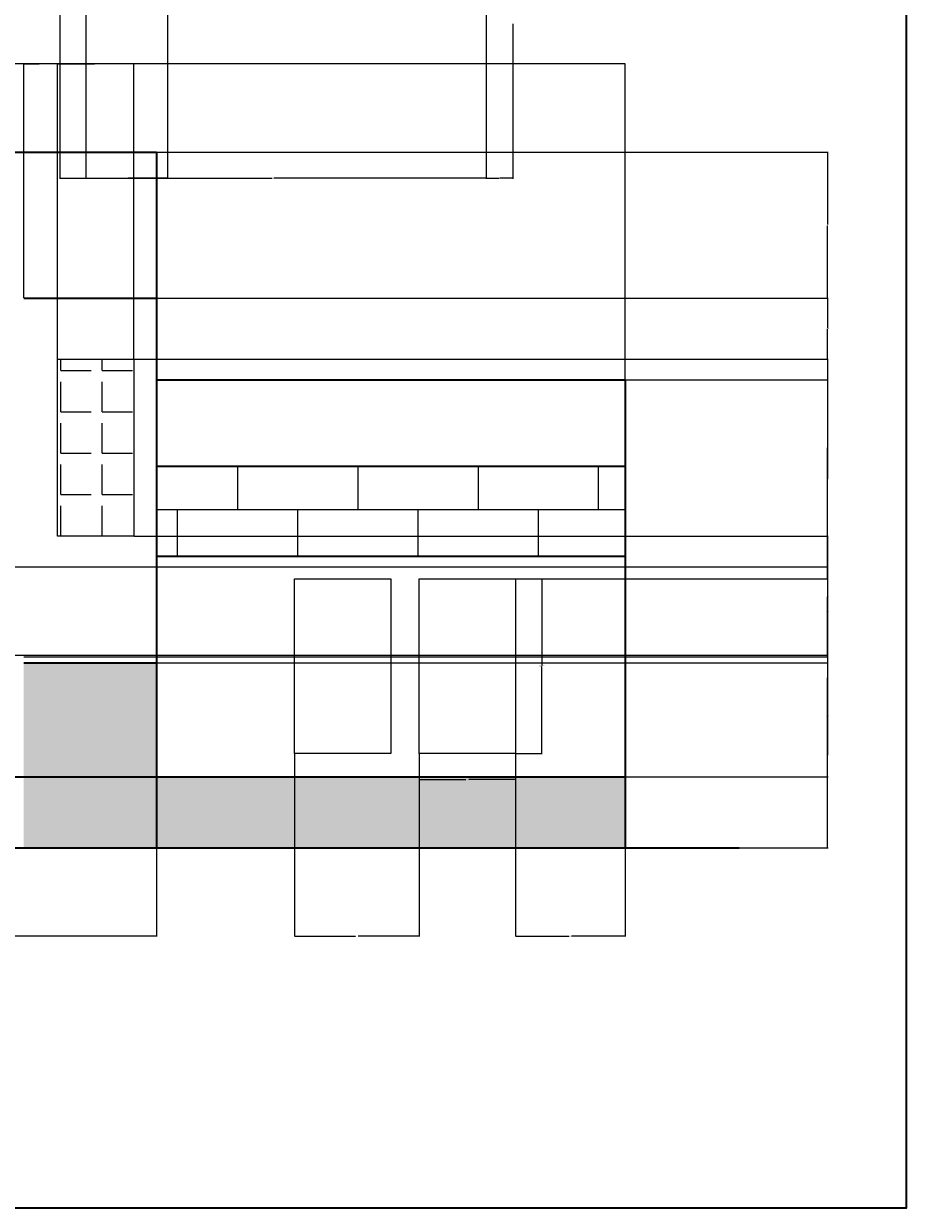
# Model space of a CAD drawing. Units: feet. Extents: x 3406 to 4127, y 2162 to 3204.
# Tile 2 of 3: x 3829 to 4127, y 2162 to 2562. Entities that reach past the tile are written whole.
import ezdxf

# ---------------------------------------------------------------- set-up
doc = ezdxf.new("R2010")
doc.units = ezdxf.units.FT
for name, color, linetype, lineweight in [('A-ANNO-DIMS', 2, 'Continuous', 18), ('A-ANNO-TTLB', 7, 'Continuous', 35), ('A-ELEV', 7, 'Continuous', 35), ('A-ELEV-GRND', 7, 'Continuous', 35), ('A-ELEV-PATT', 8, 'Continuous', 13), ('A-GLAZ', 4, 'Continuous', 25), ('A-GLAZ-PATT', 9, 'Continuous', 13)]:
    doc.layers.add(name, color=color, linetype=linetype, lineweight=lineweight)
doc.styles.get("Standard").update_dxf_attribs({"font": 'arial.ttf'})
doc.dimstyles.get("Standard").update_dxf_attribs({"dimtxt": 0.18, "dimasz": 0.18, "dimexe": 0.18, "dimexo": 0.0625, "dimgap": 0.09, "dimtad": 0, "dimtih": 1, "dimtoh": 1, "dimdec": 4, "dimzin": 0, "dimdsep": 46, "dimtxsty": 'Standard', "dimcen": 0.09, "dimadec": 0, "dimazin": 0, "dimtfac": 1, "dimtdec": 4, "dimtofl": 0, "dimtmove": 0, "dimatfit": 3, "dimfxl": 1, "dimtolj": 1, "dimtzin": 0, "dimarcsym": 0})

# ---------------------------------------------------------------- blocks, each defined once
blk = doc.blocks.new('WIN-ELEV-SINGLE')
blk.add_lwpolyline([(0, 59.01), (32.53, 59.01), (32.53, 0), (0, 0)], close=True)
blk = doc.blocks.new('*D2')
at = {"layer": 'A-ANNO-DIMS', "color": 0, "lineweight": -2, "transparency": 16777216}
for p, q in [((3995.35, 2374.42), (4004.32, 2374.42)), ((4004.14, 2374.24), (4004.14, 2345.1)), ((4004.14, 2315.6), (4004.14, 2344.74)), ((3995.35, 2315.42), (4004.32, 2315.42))]:
    blk.add_line(p, q, dxfattribs=at)
at = {"layer": 'A-ANNO-DIMS', "color": 0, "transparency": 16777216}
for points in [[(4004.11, 2374.24), (4004.17, 2374.24), (4004.14, 2374.42)], [(4004.11, 2315.6), (4004.17, 2315.6), (4004.14, 2315.42)]]:
    blk.add_solid(points, dxfattribs=at)
at = {"layer": 'Defpoints', "color": 0, "transparency": 16777216}
for p in [(3995.29, 2374.42), (4004.14, 2374.42), (3995.29, 2315.42)]:
    blk.add_point(p, dxfattribs=at)
at = {"layer": 'A-ANNO-DIMS', "color": 0, "transparency": 16777216, "insert": (4004.14, 2344.92), "char_height": 0.18, "attachment_point": 5}
blk.add_mtext('\\A1;WINDOW 59 TYP.', dxfattribs=at)
blk = doc.blocks.new('*D3')
at = {"layer": 'A-ANNO-DIMS', "color": 0, "lineweight": -2, "transparency": 16777216}
for p, q in [((3962.76, 2315.35), (3962.76, 2306.39)), ((3995.29, 2315.35), (3995.29, 2306.39)), ((3962.94, 2306.57), (3978.5, 2306.57)), ((3995.11, 2306.57), (3979.55, 2306.57))]:
    blk.add_line(p, q, dxfattribs=at)
at = {"layer": 'A-ANNO-DIMS', "color": 0, "transparency": 16777216}
for points in [[(3962.94, 2306.6), (3962.94, 2306.54), (3962.76, 2306.57)], [(3995.11, 2306.6), (3995.11, 2306.54), (3995.29, 2306.57)]]:
    blk.add_solid(points, dxfattribs=at)
at = {"layer": 'Defpoints', "color": 0, "transparency": 16777216}
for p in [(3962.76, 2315.42), (3995.29, 2315.42), (3995.29, 2306.57)]:
    blk.add_point(p, dxfattribs=at)
at = {"layer": 'A-ANNO-DIMS', "color": 0, "transparency": 16777216, "insert": (3979.03, 2306.57), "char_height": 0.18, "attachment_point": 5}
blk.add_mtext('\\A1;33 TYP.', dxfattribs=at)
blk = doc.blocks.new('*D9')
at = {"layer": 'A-ANNO-DIMS', "color": 0, "lineweight": -2, "transparency": 16777216}
for p, q in [((3841.39, 2570.84), (3841.39, 2509.54)), ((3985.39, 2570.84), (3985.39, 2509.54)), ((3841.57, 2509.72), (3913.11, 2509.72)), ((3985.21, 2509.72), (3913.67, 2509.72))]:
    blk.add_line(p, q, dxfattribs=at)
at = {"layer": 'A-ANNO-DIMS', "color": 0, "transparency": 16777216}
for points in [[(3841.57, 2509.75), (3841.57, 2509.69), (3841.39, 2509.72)], [(3985.21, 2509.75), (3985.21, 2509.69), (3985.39, 2509.72)]]:
    blk.add_solid(points, dxfattribs=at)
at = {"layer": 'Defpoints', "color": 0, "transparency": 16777216}
for p in [(3841.39, 2570.91), (3985.39, 2570.91), (3985.39, 2509.72)]:
    blk.add_point(p, dxfattribs=at)
at = {"layer": 'A-ANNO-DIMS', "color": 0, "transparency": 16777216, "insert": (3913.39, 2509.72), "char_height": 0.18, "attachment_point": 5}
blk.add_mtext('\\A1;144', dxfattribs=at)
blk = doc.blocks.new('*D16')
at = {"layer": 'A-ANNO-DIMS', "color": 0, "lineweight": -2, "transparency": 16777216}
for p, q in [((3850.19, 2904.84), (3850.19, 2509.54)), ((3877.72, 2904.84), (3877.72, 2509.54)), ((3850.37, 2509.72), (3863.49, 2509.72)), ((3877.54, 2509.72), (3864.42, 2509.72))]:
    blk.add_line(p, q, dxfattribs=at)
at = {"layer": 'A-ANNO-DIMS', "color": 0, "transparency": 16777216}
for points in [[(3850.37, 2509.75), (3850.37, 2509.69), (3850.19, 2509.72)], [(3877.54, 2509.75), (3877.54, 2509.69), (3877.72, 2509.72)]]:
    blk.add_solid(points, dxfattribs=at)
at = {"layer": 'Defpoints', "color": 0, "transparency": 16777216}
for p in [(3850.19, 2904.91), (3877.72, 2904.91), (3877.72, 2509.72)]:
    blk.add_point(p, dxfattribs=at)
at = {"layer": 'A-ANNO-DIMS', "color": 0, "transparency": 16777216, "insert": (3863.95, 2509.72), "char_height": 0.18, "attachment_point": 5}
blk.add_mtext('\\A1;27.533', dxfattribs=at)
blk = doc.blocks.new('*D22')
at = {"layer": 'A-ANNO-DIMS', "color": 0, "lineweight": -2, "transparency": 16777216}
for p, q in [((3985.39, 2570.84), (3985.39, 2509.54)), ((3994.39, 2561.84), (3994.39, 2509.54)), ((3985.57, 2509.72), (3989.74, 2509.72)), ((3994.21, 2509.72), (3990.04, 2509.72))]:
    blk.add_line(p, q, dxfattribs=at)
at = {"layer": 'A-ANNO-DIMS', "color": 0, "transparency": 16777216}
for points in [[(3985.57, 2509.75), (3985.57, 2509.69), (3985.39, 2509.72)], [(3994.21, 2509.75), (3994.21, 2509.69), (3994.39, 2509.72)]]:
    blk.add_solid(points, dxfattribs=at)
at = {"layer": 'Defpoints', "color": 0, "transparency": 16777216}
for p in [(3985.39, 2570.91), (3994.39, 2561.91), (3985.39, 2509.72)]:
    blk.add_point(p, dxfattribs=at)
at = {"layer": 'A-ANNO-DIMS', "color": 0, "transparency": 16777216, "insert": (3989.89, 2509.72), "char_height": 0.18, "attachment_point": 5}
blk.add_mtext('\\A1;9', dxfattribs=at)
blk = doc.blocks.new('*D27')
at = {"layer": 'A-ANNO-DIMS', "color": 0, "lineweight": -2, "transparency": 16777216}
for p, q in [((3561.78, 2441.65), (3561.78, 2548.49)), ((3561.96, 2548.31), (3796.68, 2548.31)), ((4032.19, 2548.31), (3797.47, 2548.31)), ((4032.37, 2441.65), (4032.37, 2548.49))]:
    blk.add_line(p, q, dxfattribs=at)
at = {"layer": 'A-ANNO-DIMS', "color": 0, "transparency": 16777216}
for points in [[(3561.96, 2548.34), (3561.96, 2548.28), (3561.78, 2548.31)], [(4032.19, 2548.34), (4032.19, 2548.28), (4032.37, 2548.31)]]:
    blk.add_solid(points, dxfattribs=at)
at = {"layer": 'Defpoints', "color": 0, "transparency": 16777216}
for p in [(4032.37, 2548.31), (3561.78, 2441.59), (4032.37, 2441.59)]:
    blk.add_point(p, dxfattribs=at)
at = {"layer": 'A-ANNO-DIMS', "color": 0, "transparency": 16777216, "insert": (3797.08, 2548.31), "char_height": 0.18, "attachment_point": 5}
blk.add_mtext('\\A1;470.6', dxfattribs=at)
blk = doc.blocks.new('*D34')
at = {"layer": 'A-ANNO-DIMS', "color": 0, "lineweight": -2, "transparency": 16777216}
for p, q in [((3747.88, 2283.42), (3747.88, 2253.51)), ((3874.08, 2283.42), (3874.08, 2253.51)), ((3748.06, 2253.69), (3810.59, 2253.69)), ((3873.9, 2253.69), (3811.36, 2253.69))]:
    blk.add_line(p, q, dxfattribs=at)
at = {"layer": 'A-ANNO-DIMS', "color": 0, "transparency": 16777216}
for points in [[(3748.06, 2253.72), (3748.06, 2253.66), (3747.88, 2253.69)], [(3873.9, 2253.72), (3873.9, 2253.66), (3874.08, 2253.69)]]:
    blk.add_solid(points, dxfattribs=at)
at = {"layer": 'Defpoints', "color": 0, "transparency": 16777216}
for p in [(3747.88, 2283.49), (3874.08, 2283.49), (3874.08, 2253.69)]:
    blk.add_point(p, dxfattribs=at)
at = {"layer": 'A-ANNO-DIMS', "color": 0, "transparency": 16777216, "insert": (3810.98, 2253.69), "char_height": 0.18, "attachment_point": 5}
blk.add_mtext('\\A1;126.2', dxfattribs=at)
blk = doc.blocks.new('*D35')
at = {"layer": 'A-ANNO-DIMS', "color": 0, "lineweight": -2, "transparency": 16777216}
for p, q in [((3920.64, 2315.35), (3920.64, 2253.51)), ((3962.76, 2315.35), (3962.76, 2253.51)), ((3920.82, 2253.69), (3941.23, 2253.69)), ((3962.58, 2253.69), (3942.17, 2253.69))]:
    blk.add_line(p, q, dxfattribs=at)
at = {"layer": 'A-ANNO-DIMS', "color": 0, "transparency": 16777216}
for points in [[(3920.82, 2253.72), (3920.82, 2253.66), (3920.64, 2253.69)], [(3962.58, 2253.72), (3962.58, 2253.66), (3962.76, 2253.69)]]:
    blk.add_solid(points, dxfattribs=at)
at = {"layer": 'Defpoints', "color": 0, "transparency": 16777216}
for p in [(3920.64, 2315.42), (3962.76, 2315.42), (3962.76, 2253.69)]:
    blk.add_point(p, dxfattribs=at)
at = {"layer": 'A-ANNO-DIMS', "color": 0, "transparency": 16777216, "insert": (3941.7, 2253.69), "char_height": 0.18, "attachment_point": 5}
blk.add_mtext('\\A1;42.125', dxfattribs=at)
blk = doc.blocks.new('*D36')
at = {"layer": 'A-ANNO-DIMS', "color": 0, "lineweight": -2, "transparency": 16777216}
for p, q in [((3995.29, 2315.35), (3995.29, 2253.51)), ((4032.37, 2283.42), (4032.37, 2253.51)), ((3995.47, 2253.69), (4013.44, 2253.69)), ((4032.19, 2253.69), (4014.22, 2253.69))]:
    blk.add_line(p, q, dxfattribs=at)
at = {"layer": 'A-ANNO-DIMS', "color": 0, "transparency": 16777216}
for points in [[(3995.47, 2253.72), (3995.47, 2253.66), (3995.29, 2253.69)], [(4032.19, 2253.72), (4032.19, 2253.66), (4032.37, 2253.69)]]:
    blk.add_solid(points, dxfattribs=at)
at = {"layer": 'Defpoints', "color": 0, "transparency": 16777216}
for p in [(3995.29, 2315.42), (4032.37, 2283.49), (4032.37, 2253.69)]:
    blk.add_point(p, dxfattribs=at)
at = {"layer": 'A-ANNO-DIMS', "color": 0, "transparency": 16777216, "insert": (4013.83, 2253.69), "char_height": 0.18, "attachment_point": 5}
blk.add_mtext('\\A1;37.08', dxfattribs=at)
blk = doc.blocks.new('*D40')
at = {"layer": 'A-ANNO-DIMS', "color": 0, "lineweight": -2, "transparency": 16777216}
for p, q in [((3995.35, 2374.42), (4100.86, 2374.42)), ((4100.68, 2374.24), (4100.68, 2341.14)), ((4100.68, 2307.68), (4100.68, 2340.78)), ((4032.43, 2307.5), (4100.86, 2307.5))]:
    blk.add_line(p, q, dxfattribs=at)
at = {"layer": 'A-ANNO-DIMS', "color": 0, "transparency": 16777216}
for points in [[(4100.65, 2374.24), (4100.71, 2374.24), (4100.68, 2374.42)], [(4100.65, 2307.68), (4100.71, 2307.68), (4100.68, 2307.5)]]:
    blk.add_solid(points, dxfattribs=at)
at = {"layer": 'Defpoints', "color": 0, "transparency": 16777216}
for p in [(3995.29, 2374.42), (4100.68, 2374.42), (4032.37, 2307.5)]:
    blk.add_point(p, dxfattribs=at)
at = {"layer": 'A-ANNO-DIMS', "color": 0, "transparency": 16777216, "insert": (4100.68, 2340.96), "char_height": 0.18, "attachment_point": 5}
blk.add_mtext('\\A1;66.93', dxfattribs=at)
blk = doc.blocks.new('*D41')
at = {"layer": 'A-ANNO-DIMS', "color": 0, "lineweight": -2, "transparency": 16777216}
for p, q in [((4032.43, 2441.59), (4100.86, 2441.59)), ((4100.68, 2441.41), (4100.68, 2408.19)), ((4100.68, 2374.6), (4100.68, 2407.83)), ((3995.35, 2374.42), (4100.86, 2374.42))]:
    blk.add_line(p, q, dxfattribs=at)
at = {"layer": 'A-ANNO-DIMS', "color": 0, "transparency": 16777216}
for points in [[(4100.65, 2441.41), (4100.71, 2441.41), (4100.68, 2441.59)], [(4100.65, 2374.6), (4100.71, 2374.6), (4100.68, 2374.42)]]:
    blk.add_solid(points, dxfattribs=at)
at = {"layer": 'Defpoints', "color": 0, "transparency": 16777216}
for p in [(4032.37, 2441.59), (4100.68, 2441.59), (3995.29, 2374.42)]:
    blk.add_point(p, dxfattribs=at)
at = {"layer": 'A-ANNO-DIMS', "color": 0, "transparency": 16777216, "insert": (4100.68, 2408.01), "char_height": 0.18, "attachment_point": 5}
blk.add_mtext('\\A1;67.17', dxfattribs=at)
blk = doc.blocks.new('*D42')
at = {"layer": 'A-ANNO-DIMS', "color": 0, "lineweight": -2, "transparency": 16777216}
for p, q in [((3644.1, 2378.49), (4100.86, 2378.49)), ((4100.68, 2378.31), (4100.68, 2363.7)), ((4100.68, 2348.73), (4100.68, 2363.34)), ((3644.1, 2348.55), (4100.86, 2348.55))]:
    blk.add_line(p, q, dxfattribs=at)
at = {"layer": 'A-ANNO-DIMS', "color": 0, "transparency": 16777216}
for points in [[(4100.65, 2378.31), (4100.71, 2378.31), (4100.68, 2378.49)], [(4100.65, 2348.73), (4100.71, 2348.73), (4100.68, 2348.55)]]:
    blk.add_solid(points, dxfattribs=at)
at = {"layer": 'Defpoints', "color": 0, "transparency": 16777216}
for p in [(3644.04, 2378.49), (4100.68, 2378.49), (3644.04, 2348.55)]:
    blk.add_point(p, dxfattribs=at)
at = {"layer": 'A-ANNO-DIMS', "color": 0, "transparency": 16777216, "insert": (4100.68, 2363.52), "char_height": 0.18, "attachment_point": 5}
blk.add_mtext('\\A1;29.935', dxfattribs=at)
blk = doc.blocks.new('*D43')
at = {"layer": 'A-ANNO-DIMS', "color": 0, "lineweight": -2, "transparency": 16777216}
for p, q in [((3644.1, 2348.55), (4100.86, 2348.55)), ((4100.68, 2348.37), (4100.68, 2328.21)), ((4100.68, 2307.68), (4100.68, 2327.84)), ((3674.17, 2307.5), (4100.86, 2307.5))]:
    blk.add_line(p, q, dxfattribs=at)
at = {"layer": 'A-ANNO-DIMS', "color": 0, "transparency": 16777216}
for points in [[(4100.65, 2348.37), (4100.71, 2348.37), (4100.68, 2348.55)], [(4100.65, 2307.68), (4100.71, 2307.68), (4100.68, 2307.5)]]:
    blk.add_solid(points, dxfattribs=at)
at = {"layer": 'Defpoints', "color": 0, "transparency": 16777216}
for p in [(3644.04, 2348.55), (3674.11, 2307.5), (4100.68, 2307.5)]:
    blk.add_point(p, dxfattribs=at)
at = {"layer": 'A-ANNO-DIMS', "color": 0, "transparency": 16777216, "insert": (4100.68, 2328.02), "char_height": 0.18, "attachment_point": 5}
blk.add_mtext('\\A1;41.055', dxfattribs=at)
blk = doc.blocks.new('*D45')
at = {"layer": 'A-ANNO-DIMS', "color": 0, "lineweight": -2, "transparency": 16777216}
for p, q in [((3795.84, 2484.91), (3795.84, 2548.49)), ((3796.02, 2548.31), (3812.11, 2548.31)), ((3828.99, 2548.31), (3812.9, 2548.31)), ((3829.17, 2469.25), (3829.17, 2548.49))]:
    blk.add_line(p, q, dxfattribs=at)
at = {"layer": 'A-ANNO-DIMS', "color": 0, "transparency": 16777216}
for points in [[(3796.02, 2548.34), (3796.02, 2548.28), (3795.84, 2548.31)], [(3828.99, 2548.34), (3828.99, 2548.28), (3829.17, 2548.31)]]:
    blk.add_solid(points, dxfattribs=at)
at = {"layer": 'Defpoints', "color": 0, "transparency": 16777216}
for p in [(3829.17, 2548.31), (3795.84, 2484.85), (3829.17, 2469.19)]:
    blk.add_point(p, dxfattribs=at)
at = {"layer": 'A-ANNO-DIMS', "color": 0, "transparency": 16777216, "insert": (3812.51, 2548.31), "char_height": 0.18, "attachment_point": 5}
blk.add_mtext('\\A1;33.32', dxfattribs=at)
blk = doc.blocks.new('*D50')
at = {"layer": 'A-ANNO-DIMS', "color": 0, "lineweight": -2, "transparency": 16777216}
for p, q in [((3829.17, 2469.25), (3829.17, 2548.49)), ((3829.35, 2548.31), (3834.43, 2548.31)), ((3840.42, 2548.31), (3835.34, 2548.31)), ((3840.6, 2448.6), (3840.6, 2548.49))]:
    blk.add_line(p, q, dxfattribs=at)
at = {"layer": 'A-ANNO-DIMS', "color": 0, "transparency": 16777216}
for points in [[(3829.35, 2548.34), (3829.35, 2548.28), (3829.17, 2548.31)], [(3840.42, 2548.34), (3840.42, 2548.28), (3840.6, 2548.31)]]:
    blk.add_solid(points, dxfattribs=at)
at = {"layer": 'Defpoints', "color": 0, "transparency": 16777216}
for p in [(3840.6, 2548.31), (3829.17, 2469.19), (3840.6, 2448.54)]:
    blk.add_point(p, dxfattribs=at)
at = {"layer": 'A-ANNO-DIMS', "color": 0, "transparency": 16777216, "insert": (3834.88, 2548.31), "char_height": 0.18, "attachment_point": 5}
blk.add_mtext('\\A1;11.434', dxfattribs=at)
blk = doc.blocks.new('*D51')
at = {"layer": 'A-ANNO-DIMS', "color": 0, "lineweight": -2, "transparency": 16777216}
for p, q in [((3840.6, 2448.6), (3840.6, 2548.49)), ((3840.78, 2548.31), (3853.05, 2548.31)), ((3866.24, 2548.31), (3853.98, 2548.31)), ((3866.42, 2448.6), (3866.42, 2548.49))]:
    blk.add_line(p, q, dxfattribs=at)
at = {"layer": 'A-ANNO-DIMS', "color": 0, "transparency": 16777216}
for points in [[(3840.78, 2548.34), (3840.78, 2548.28), (3840.6, 2548.31)], [(3866.24, 2548.34), (3866.24, 2548.28), (3866.42, 2548.31)]]:
    blk.add_solid(points, dxfattribs=at)
at = {"layer": 'Defpoints', "color": 0, "transparency": 16777216}
for p in [(3866.42, 2548.31), (3840.6, 2448.54), (3866.42, 2448.54)]:
    blk.add_point(p, dxfattribs=at)
at = {"layer": 'A-ANNO-DIMS', "color": 0, "transparency": 16777216, "insert": (3853.51, 2548.31), "char_height": 0.18, "attachment_point": 5}
blk.add_mtext('\\A1;25.823', dxfattribs=at)
blk = doc.blocks.new('*D56')
at = {"layer": 'A-ANNO-DIMS', "color": 0, "lineweight": -2, "transparency": 16777216}
for p, q in [((3874.14, 2518.51), (4100.86, 2518.51)), ((4100.68, 2518.33), (4100.68, 2494.03)), ((4100.68, 2469.37), (4100.68, 2493.67)), ((3874.14, 2469.19), (4100.86, 2469.19))]:
    blk.add_line(p, q, dxfattribs=at)
at = {"layer": 'A-ANNO-DIMS', "color": 0, "transparency": 16777216}
for points in [[(4100.65, 2518.33), (4100.71, 2518.33), (4100.68, 2518.51)], [(4100.65, 2469.37), (4100.71, 2469.37), (4100.68, 2469.19)]]:
    blk.add_solid(points, dxfattribs=at)
at = {"layer": 'Defpoints', "color": 0, "transparency": 16777216}
for p in [(3874.08, 2518.51), (3874.08, 2469.19), (4100.68, 2469.19)]:
    blk.add_point(p, dxfattribs=at)
at = {"layer": 'A-ANNO-DIMS', "color": 0, "transparency": 16777216, "insert": (4100.68, 2493.85), "char_height": 0.18, "attachment_point": 5}
blk.add_mtext('\\A1;49.32', dxfattribs=at)
blk = doc.blocks.new('*D57')
at = {"layer": 'A-ANNO-DIMS', "color": 0, "lineweight": -2, "transparency": 16777216}
for p, q in [((3874.14, 2469.19), (4100.86, 2469.19)), ((4100.68, 2469.01), (4100.68, 2459.05)), ((4100.68, 2448.72), (4100.68, 2458.68)), ((3866.49, 2448.54), (4100.86, 2448.54))]:
    blk.add_line(p, q, dxfattribs=at)
at = {"layer": 'A-ANNO-DIMS', "color": 0, "transparency": 16777216}
for points in [[(4100.65, 2469.01), (4100.71, 2469.01), (4100.68, 2469.19)], [(4100.65, 2448.72), (4100.71, 2448.72), (4100.68, 2448.54)]]:
    blk.add_solid(points, dxfattribs=at)
at = {"layer": 'Defpoints', "color": 0, "transparency": 16777216}
for p in [(3874.08, 2469.19), (3866.42, 2448.54), (4100.68, 2448.54)]:
    blk.add_point(p, dxfattribs=at)
at = {"layer": 'A-ANNO-DIMS', "color": 0, "transparency": 16777216, "insert": (4100.68, 2458.86), "char_height": 0.18, "attachment_point": 5}
blk.add_mtext('\\A1;20.654', dxfattribs=at)
blk = doc.blocks.new('*D58')
at = {"layer": 'A-ANNO-DIMS', "color": 0, "lineweight": -2, "transparency": 16777216}
for p, q in [((3866.49, 2448.54), (4100.86, 2448.54)), ((4100.68, 2448.36), (4100.68, 2418.85)), ((4100.68, 2388.98), (4100.68, 2418.49)), ((3866.49, 2388.8), (4100.86, 2388.8))]:
    blk.add_line(p, q, dxfattribs=at)
at = {"layer": 'A-ANNO-DIMS', "color": 0, "transparency": 16777216}
for points in [[(4100.65, 2448.36), (4100.71, 2448.36), (4100.68, 2448.54)], [(4100.65, 2388.98), (4100.71, 2388.98), (4100.68, 2388.8)]]:
    blk.add_solid(points, dxfattribs=at)
at = {"layer": 'Defpoints', "color": 0, "transparency": 16777216}
for p in [(3866.42, 2448.54), (3866.42, 2388.8), (4100.68, 2388.8)]:
    blk.add_point(p, dxfattribs=at)
at = {"layer": 'A-ANNO-DIMS', "color": 0, "transparency": 16777216, "insert": (4100.68, 2418.67), "char_height": 0.18, "attachment_point": 5}
blk.add_mtext('\\A1;59.74', dxfattribs=at)
blk = doc.blocks.new('*D59')
at = {"layer": 'A-ANNO-DIMS', "color": 0, "lineweight": -2, "transparency": 16777216}
for p, q in [((3866.49, 2388.8), (4100.86, 2388.8)), ((4100.68, 2388.62), (4100.68, 2368.59)), ((4100.68, 2348.19), (4100.68, 2368.22)), ((3829.23, 2348.01), (4100.86, 2348.01))]:
    blk.add_line(p, q, dxfattribs=at)
at = {"layer": 'A-ANNO-DIMS', "color": 0, "transparency": 16777216}
for points in [[(4100.65, 2388.62), (4100.71, 2388.62), (4100.68, 2388.8)], [(4100.65, 2348.19), (4100.71, 2348.19), (4100.68, 2348.01)]]:
    blk.add_solid(points, dxfattribs=at)
at = {"layer": 'Defpoints', "color": 0, "transparency": 16777216}
for p in [(3866.42, 2388.8), (3829.17, 2348.01), (4100.68, 2348.01)]:
    blk.add_point(p, dxfattribs=at)
at = {"layer": 'A-ANNO-DIMS', "color": 0, "transparency": 16777216, "insert": (4100.68, 2368.4), "char_height": 0.18, "attachment_point": 5}
blk.add_mtext('\\A1;40.786', dxfattribs=at)
blk = doc.blocks.new('*D60')
at = {"layer": 'A-ANNO-DIMS', "color": 0, "lineweight": -2, "transparency": 16777216}
for p, q in [((3874.14, 2345.98), (4100.86, 2345.98)), ((4100.68, 2345.8), (4100.68, 2314.92)), ((4100.68, 2283.67), (4100.68, 2314.55)), ((3874.14, 2283.49), (4100.86, 2283.49))]:
    blk.add_line(p, q, dxfattribs=at)
at = {"layer": 'A-ANNO-DIMS', "color": 0, "transparency": 16777216}
for points in [[(4100.65, 2345.8), (4100.71, 2345.8), (4100.68, 2345.98)], [(4100.65, 2283.67), (4100.71, 2283.67), (4100.68, 2283.49)]]:
    blk.add_solid(points, dxfattribs=at)
at = {"layer": 'Defpoints', "color": 0, "transparency": 16777216}
for p in [(3874.08, 2345.98), (4100.68, 2345.98), (3874.08, 2283.49)]:
    blk.add_point(p, dxfattribs=at)
at = {"layer": 'A-ANNO-DIMS', "color": 0, "transparency": 16777216, "insert": (4100.68, 2314.74), "char_height": 0.18, "attachment_point": 5}
blk.add_mtext('\\A1;62.5', dxfattribs=at)

msp = doc.modelspace()

# ---------------------------------------------------------------- hatches: boundary and pattern name
at = {"layer": 'A-ELEV-PATT'}
h = msp.add_hatch(dxfattribs=at)
h.set_pattern_fill('AR-B816', color=256, scale=0.1)
h.paths.add_polyline_path([(3747.8769, 2409.819), (3561.7785, 2409.819), (3561.7785, 2382.0333), (3747.8769, 2382.0333)])
h.paths.add_polyline_path([(4032.3722, 2412.4251), (3874.0816, 2412.4251), (3874.0816, 2382.0333), (4032.3722, 2382.0333)])
h = msp.add_hatch(dxfattribs=at)
h.set_pattern_fill('BRICK', color=256, scale=0.5)
h.paths.add_polyline_path([(3874.0816, 2345.984), (3829.1663, 2345.984), (3829.1663, 2307.4958), (3874.0816, 2307.4958)])
h.paths.add_polyline_path([(3874.0816, 2307.4958), (3829.1663, 2307.4958), (3829.1663, 2283.4863), (3874.0816, 2283.4863)])
h.paths.add_polyline_path([(4032.3722, 2307.4958), (3874.0816, 2307.4958), (3874.0816, 2283.4863), (4032.3722, 2283.4863)])
h.paths.add_polyline_path([(3682.9714, 2307.4958), (3561.7785, 2307.4958), (3561.7785, 2283.4863), (3682.9714, 2283.4863)])
at = {"layer": 'A-GLAZ-PATT'}
h = msp.add_hatch(dxfattribs=at)
h.set_pattern_fill('ANGLE', color=256, scale=2)
h.set_pattern_definition([(0, (0, 0), (0, 13.97), [10.16, -3.81]), (90, (0, 0), (-13.97, 9e-16), [10.16, -3.81])])
h.paths.add_polyline_path([(3866.4229, 2448.5363), (3840.6, 2448.5363), (3840.6, 2388.7978), (3866.4229, 2388.7978)])
h.paths.add_polyline_path([(3821.3093, 2448.5363), (3804.5796, 2455.082), (3804.5796, 2392.5307), (3821.3093, 2385.0649)])
h.paths.add_polyline_path([(3785.0653, 2455.082), (3765.6683, 2455.082), (3765.6683, 2392.5307), (3785.0653, 2392.5307)])

# ---------------------------------------------------------------- linework, layer by layer
at = {"layer": 'A-ANNO-TTLB'}
msp.add_lwpolyline([(3405.6917, 3203.7208), (4127.2965, 3203.7208), (4127.2965, 2161.7472), (3405.6917, 2161.7472)], close=True, dxfattribs=at)
at = {"layer": 'A-ELEV'}
for p, q in [((3747.8769, 2518.5088), (3874.0816, 2518.5088)), ((3874.0816, 2518.5088), (3874.0816, 2283.4863)), ((3829.1663, 2469.1901), (3874.0816, 2469.1901)), ((3874.0816, 2441.5924), (4032.3722, 2441.5924)), ((4032.3722, 2441.5924), (4032.3722, 2283.4863)), ((3874.0816, 2412.4251), (4032.3722, 2412.4251)), ((3874.0816, 2382.0333), (4032.3722, 2382.0333)), ((3829.1663, 2345.984), (3874.0816, 2345.984)), ((3561.7785, 2307.4958), (4032.3722, 2307.4958))]:
    msp.add_line(p, q, dxfattribs=at)
at = {"layer": 'A-ELEV-GRND'}
msp.add_line((3561.7785, 2283.4863), (4070.8753, 2283.4863), dxfattribs=at)
at = {"layer": 'A-GLAZ'}
for p, q in [((3840.6, 2448.5363), (3866.4229, 2448.5363)), ((3840.6, 2388.7978), (3840.6, 2448.5363)), ((3866.4229, 2448.5363), (3866.4229, 2388.7978)), ((3866.4229, 2388.7978), (3840.6, 2388.7978))]:
    msp.add_line(p, q, dxfattribs=at)

# ---------------------------------------------------------------- block references
for p in [(3920.638, 2315.416), (3962.7633, 2315.416)]:
    msp.add_blockref('WIN-ELEV-SINGLE', p, dxfattribs=at)

# ---------------------------------------------------------------- dimensions: what is measured, and where the dimension line sits
at = {"layer": 'A-ANNO-DIMS'}
for base, p1, p2, override, picture, middle in [((3877.7214, 2509.7223), (3850.1884, 2904.9057), (3877.7214, 2904.9057), {"dimdec": 3, "dimlfac": 1, "dimrnd": 0, "dimzin": 0, "dimdsep": 46, "dimlunit": 2}, '*D16', (3863.9549, 2509.7223)), ((3985.3916, 2509.7223), (3841.3916, 2570.9057), (3985.3916, 2570.9057), {"dimdec": 0, "dimlfac": 1, "dimrnd": 0, "dimzin": 0, "dimdsep": 46, "dimlunit": 2}, '*D9', (3913.3916, 2509.7223)), ((3985.3916, 2509.7223), (3994.3916, 2561.9057), (3985.3916, 2570.9057), {"dimdec": 0, "dimlfac": 1, "dimrnd": 0, "dimzin": 0, "dimdsep": 46, "dimlunit": 2}, '*D22', (3989.8916, 2509.7223)), ((4032.3722, 2548.3088), (3561.7785, 2441.5924), (4032.3722, 2441.5924), {"dimdec": 1, "dimlfac": 1, "dimrnd": 0, "dimzin": 0, "dimdsep": 46, "dimlunit": 2}, '*D27', (3797.0754, 2548.3088)), ((3829.1663, 2548.3088), (3795.8441, 2484.8499), (3829.1663, 2469.1901), {"dimdec": 2, "dimlfac": 1, "dimrnd": 0, "dimzin": 0, "dimdsep": 46, "dimlunit": 2}, '*D45', (3812.5052, 2548.3088)), ((3840.6, 2548.3088), (3829.1663, 2469.1901), (3840.6, 2448.5363), {"dimdec": 3, "dimlfac": 1, "dimrnd": 0, "dimzin": 0, "dimdsep": 46, "dimlunit": 2}, '*D50', (3834.8831, 2548.3088)), ((3866.4229, 2548.3088), (3840.6, 2448.5363), (3866.4229, 2448.5363), {"dimdec": 3, "dimlfac": 1, "dimrnd": 0, "dimzin": 0, "dimdsep": 46, "dimlunit": 2}, '*D51', (3853.5114, 2548.3088)), ((3962.763, 2253.6863), (3920.6377, 2315.4164), (3962.763, 2315.4164), {"dimdec": 3, "dimlfac": 1, "dimrnd": 0, "dimzin": 0, "dimdsep": 46, "dimlunit": 2}, '*D35', (3941.7003, 2253.6863)), ((4032.3722, 2253.6863), (3995.2901, 2315.4164), (4032.3722, 2283.4863), {"dimdec": 2, "dimlfac": 1, "dimrnd": 0, "dimzin": 0, "dimdsep": 46, "dimlunit": 2}, '*D36', (4013.8312, 2253.6863)), ((3874.0816, 2253.6863), (3747.8769, 2283.4863), (3874.0816, 2283.4863), {"dimdec": 1, "dimlfac": 1, "dimrnd": 0, "dimzin": 0, "dimdsep": 46, "dimlunit": 2}, '*D34', (3810.9793, 2253.6863))]:
    dim = msp.add_linear_dim(base=base, p1=p1, p2=p2, dimstyle='Standard', override=override, dxfattribs=at)
    dim.commit()
    dim.dimension.update_dxf_attribs({"geometry": picture, "text_midpoint": middle})
for base, p1, p2, override, picture, middle in [((4100.6753, 2469.1901), (3874.0816, 2518.5088), (3874.0816, 2469.1901), {"dimdec": 2, "dimlfac": 1, "dimrnd": 0, "dimzin": 0, "dimdsep": 46, "dimlunit": 2}, '*D56', (4100.6753, 2493.8495)), ((4100.6753, 2448.5363), (3874.0816, 2469.1901), (3866.4229, 2448.5363), {"dimdec": 3, "dimlfac": 1, "dimrnd": 0, "dimzin": 0, "dimdsep": 46, "dimlunit": 2}, '*D57', (4100.6753, 2458.8632)), ((4100.6753, 2388.7978), (3866.4229, 2448.5363), (3866.4229, 2388.7978), {"dimdec": 2, "dimlfac": 1, "dimrnd": 0, "dimzin": 0, "dimdsep": 46, "dimlunit": 2}, '*D58', (4100.6753, 2418.667)), ((4100.6753, 2441.5924), (3995.2901, 2374.4234), (4032.3722, 2441.5924), {"dimdec": 2, "dimlfac": 1, "dimrnd": 0, "dimzin": 0, "dimdsep": 46, "dimlunit": 2}, '*D41', (4100.6753, 2408.0079)), ((4100.6753, 2348.012), (3866.4229, 2388.7978), (3829.1663, 2348.012), {"dimdec": 3, "dimlfac": 1, "dimrnd": 0, "dimzin": 0, "dimdsep": 46, "dimlunit": 2}, '*D59', (4100.6753, 2368.4049)), ((4100.67532, 2378.4862), (3644.0412, 2348.55074), (3644.0412, 2378.4862), {"dimdec": 3, "dimlfac": 1, "dimrnd": 0, "dimzin": 0, "dimdsep": 46, "dimlunit": 2}, '*D42', (4100.67532, 2363.51847)), ((4100.6753, 2374.4234), (4032.3722, 2307.4958), (3995.2901, 2374.4234), {"dimdec": 2, "dimlfac": 1, "dimrnd": 0, "dimzin": 0, "dimdsep": 46, "dimlunit": 2}, '*D40', (4100.6753, 2340.9596)), ((4100.6753, 2307.4958), (3644.0412, 2348.5507), (3674.1115, 2307.4958), {"dimdec": 3, "dimlfac": 1, "dimrnd": 0, "dimzin": 0, "dimdsep": 46, "dimlunit": 2}, '*D43', (4100.6753, 2328.0233)), ((4100.6753, 2345.984), (3874.0816, 2283.4863), (3874.0816, 2345.984), {"dimdec": 1, "dimlfac": 1, "dimrnd": 0, "dimzin": 0, "dimdsep": 46, "dimlunit": 2}, '*D60', (4100.6753, 2314.7351))]:
    dim = msp.add_linear_dim(base=base, p1=p1, p2=p2, angle=90, dimstyle='Standard', override=override, dxfattribs=at)
    dim.commit()
    dim.dimension.update_dxf_attribs({"geometry": picture, "text_midpoint": middle})
dim = msp.add_linear_dim(base=(4004.1412, 2374.4234), p1=(3995.2901, 2315.4164), p2=(3995.2901, 2374.4234), angle=90, text='WINDOW <> TYP.', dimstyle='Standard', override={"dimdec": 0, "dimlfac": 1, "dimrnd": 0, "dimzin": 0, "dimdsep": 46, "dimlunit": 2}, dxfattribs=at)
dim.commit()
dim.dimension.update_dxf_attribs({"geometry": '*D2', "text_midpoint": (4004.1412, 2344.9199)})
dim = msp.add_linear_dim(base=(3995.2901, 2306.5653), p1=(3962.763, 2315.4164), p2=(3995.2901, 2315.4164), text='<> TYP.', dimstyle='Standard', override={"dimdec": 0, "dimlfac": 1, "dimrnd": 0, "dimzin": 0, "dimdsep": 46, "dimlunit": 2}, dxfattribs=at)
dim.commit()
dim.dimension.update_dxf_attribs({"geometry": '*D3', "text_midpoint": (3979.0265, 2306.5653)})

doc.saveas('drawing.dxf')
